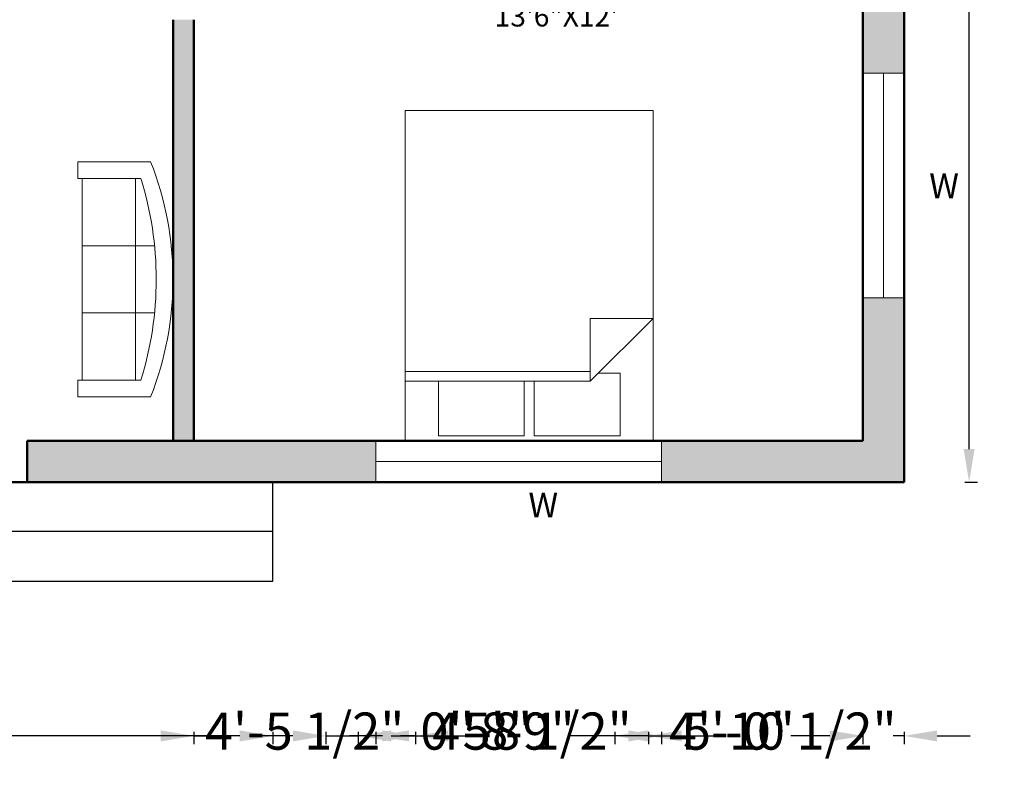
# Model space of a CAD drawing. Units: inches. Extents: x 2568 to 3190, y 746 to 1467.
# Tile 3 of 7: x 2900 to 3139, y 746 to 933. Entities that reach past the tile are written whole.
import ezdxf

# ---------------------------------------------------------------- set-up
doc = ezdxf.new("R2010")
doc.units = ezdxf.units.IN
for name, color, linetype, lineweight in [('A-ANNO-DIMS', 2, 'Continuous', 18), ('A-ANNO-TEXT', 7, 'Continuous', 18), ('A-AREA-IDEN', 7, 'Continuous', 25), ('A-FLOR-STRS', 7, 'Continuous', 25), ('A-FURN', 8, 'Continuous', 18), ('A-GLAZ', 4, 'Continuous', 20), ('A-WALL', 7, 'Continuous', 50), ('A-WALL-PATT', 252, 'Continuous', 13)]:
    doc.layers.add(name, color=color, linetype=linetype, lineweight=lineweight)
doc.styles.get("Standard").update_dxf_attribs({"font": 'arial.ttf'})
doc.dimstyles.new('ISO-25', dxfattribs={"dimtxt": 9, "dimasz": 8, "dimexe": 2, "dimexo": 1, "dimtad": 0, "dimtih": 1, "dimtoh": 1, "dimdec": 1, "dimlunit": 3, "dimtxsty": 'Standard', "dimcen": 2.5, "dimclrd": 1, "dimclre": 3, "dimclrt": 6, "dimadec": 0, "dimazin": 0, "dimtfac": 1, "dimtdec": 1, "dimtmove": 0, "dimatfit": 3, "dimfxl": 1, "dimfxlon": 1, "dimarcsym": 0})

# ---------------------------------------------------------------- blocks, each defined once
blk = doc.blocks.new('Bed - Queen')
for p, q in [((0, -80.00003), (0, 0)), ((0, 0), (59.99999, 0)), ((59.99999, 0), (59.99999, -80.00003)), ((7.99999, -1.2), (28.79998, -1.2)), ((7.99999, -14.4), (7.99999, -1.2)), ((28.79998, -1.2), (28.79998, -14.4)), ((31.19999, -1.2), (51.99999, -1.2)), ((31.19999, -14.4), (31.19999, -1.2)), ((51.99999, -1.2), (51.99999, -16.4)), ((0, -14.4), (44.8, -14.4)), ((59.99999, -29.6), (44.8, -14.4)), ((44.8, -14.4), (44.8, -29.6)), ((51.99999, -16.4), (46.79936, -16.4)), ((44.8, -16.8), (0, -16.8)), ((44.8, -29.6), (59.99999, -29.6)), ((59.99999, -80.00003), (0, -80.00003))]:
    blk.add_line(p, q)
blk = doc.blocks.new('Sofa - Roundback 7 ft.')
for p, q in [((-12.00002, -32.4421), (-12.00003, -6.5971)), ((11.99997, -32.4421), (11.99998, -6.5971)), ((-36.000027, -34), (-36.000027, -11.4696)), ((-35.999844, -13.3819), (35.9998, -13.3819)), ((35.99998, -34), (35.99998, -11.4696)), ((-36.000027, -32.4421), (35.99998, -32.4421))]:
    blk.add_line(p, q)
for points in [[(-36.000027, -34), (-42.000027, -34), (-42.000027, -8)], [(41.99998, -8), (41.99998, -34), (35.99998, -34)]]:
    blk.add_lwpolyline(points)
for centre, radius, start, end in [((0, -114.25), 114.25, 68.43141, 111.5686), ((-0.00001, -127.1968), 121.1968, 72.72033, 107.2797)]:
    blk.add_arc(centre, radius, start, end)
blk = doc.blocks.new('*D14')
at = {"layer": 'A-ANNO-DIMS', "color": 0, "lineweight": -2, "transparency": 16777216}
for p, q in [((3129.28, 1421.35), (3132.28, 1421.35)), ((3130.28, 1413.35), (3130.28, 1126.57)), ((3130.28, 829.35), (3130.28, 1116.13)), ((3129.28, 821.35), (3132.28, 821.35))]:
    blk.add_line(p, q, dxfattribs=at)
at = {"layer": 'A-ANNO-DIMS', "color": 0, "transparency": 16777216}
for points in [[(3128.95, 1413.35), (3131.61, 1413.35), (3130.28, 1421.35)], [(3128.95, 829.35), (3131.61, 829.35), (3130.28, 821.35)]]:
    blk.add_solid(points, dxfattribs=at)
at = {"layer": 'Defpoints', "color": 0, "transparency": 16777216}
for p in [(3114.52, 1421.35), (3114.52, 821.35), (3130.28, 821.35)]:
    blk.add_point(p, dxfattribs=at)
at = {"layer": 'A-ANNO-DIMS', "color": 0, "transparency": 16777216, "insert": (3130.28, 1121.35), "char_height": 9, "attachment_point": 5}
blk.add_mtext("50'", dxfattribs=at)
blk = doc.blocks.new('WIN-BED-LOWER-54.48')
for p, q in [((-5, 54.48), (5, 54.48)), ((0, 0), (0, 54.48)), ((5, 0), (-5, 0))]:
    blk.add_line(p, q)
blk = doc.blocks.new('*D43')
at = {"layer": 'A-ANNO-DIMS', "color": 3, "lineweight": -2, "transparency": 16777216}
for p, q in [((2942.52, 760.85), (2942.52, 757.85)), ((2996.2, 760.85), (2996.2, 757.85))]:
    blk.add_line(p, q, dxfattribs=at)
at = {"layer": 'A-ANNO-DIMS', "color": 1, "lineweight": -2, "transparency": 16777216}
for p, q in [((2934.52, 759.85), (2926.52, 759.85)), ((2942.52, 759.85), (2946.11, 759.85)), ((2996.2, 759.85), (2992.62, 759.85)), ((3004.2, 759.85), (3012.2, 759.85))]:
    blk.add_line(p, q, dxfattribs=at)
at = {"layer": 'A-ANNO-DIMS', "color": 1, "transparency": 16777216}
for points in [[(2934.52, 761.18), (2934.52, 758.51), (2942.52, 759.85)], [(3004.2, 761.18), (3004.2, 758.51), (2996.2, 759.85)]]:
    blk.add_solid(points, dxfattribs=at)
at = {"layer": 'Defpoints', "color": 0, "transparency": 16777216}
for p in [(2942.52, 1411.35), (2996.2, 1411.35), (2996.2, 759.85)]:
    blk.add_point(p, dxfattribs=at)
at = {"layer": 'A-ANNO-DIMS', "color": 6, "transparency": 16777216, "insert": (2969.36, 759.85), "char_height": 9, "attachment_point": 5}
blk.add_mtext('4\'-5 1/2"', dxfattribs=at)
blk = doc.blocks.new('*D44')
at = {"layer": 'A-ANNO-DIMS', "color": 3, "lineweight": -2, "transparency": 16777216}
for p, q in [((2996.2, 760.85), (2996.2, 757.85)), ((3052.64, 760.85), (3052.64, 757.85))]:
    blk.add_line(p, q, dxfattribs=at)
at = {"layer": 'A-ANNO-DIMS', "color": 1, "lineweight": -2, "transparency": 16777216}
for p, q in [((2988.2, 759.85), (2980.2, 759.85)), ((2996.2, 759.85), (3001.17, 759.85)), ((3052.64, 759.85), (3047.67, 759.85)), ((3060.64, 759.85), (3068.64, 759.85))]:
    blk.add_line(p, q, dxfattribs=at)
at = {"layer": 'A-ANNO-DIMS', "color": 1, "transparency": 16777216}
for points in [[(2988.2, 761.18), (2988.2, 758.51), (2996.2, 759.85)], [(3060.64, 761.18), (3060.64, 758.51), (3052.64, 759.85)]]:
    blk.add_solid(points, dxfattribs=at)
at = {"layer": 'Defpoints', "color": 0, "transparency": 16777216}
for p in [(2996.2, 1411.35), (3052.64, 1411.35), (3052.64, 759.85)]:
    blk.add_point(p, dxfattribs=at)
at = {"layer": 'A-ANNO-DIMS', "color": 6, "transparency": 16777216, "insert": (3024.42, 759.85), "char_height": 9, "attachment_point": 5}
blk.add_mtext('4\'-8 1/2"', dxfattribs=at)
blk = doc.blocks.new('*D48')
at = {"layer": 'A-ANNO-DIMS', "color": 3, "lineweight": -2, "transparency": 16777216}
for p, q in [((2986.63, 760.85), (2986.63, 757.85)), ((3055.78, 760.85), (3055.78, 757.85))]:
    blk.add_line(p, q, dxfattribs=at)
at = {"layer": 'A-ANNO-DIMS', "color": 1, "lineweight": -2, "transparency": 16777216}
for p, q in [((2994.63, 759.85), (3008.62, 759.85)), ((3047.78, 759.85), (3033.79, 759.85))]:
    blk.add_line(p, q, dxfattribs=at)
at = {"layer": 'A-ANNO-DIMS', "color": 1, "transparency": 16777216}
for points in [[(2994.63, 761.18), (2994.63, 758.51), (2986.63, 759.85)], [(3047.78, 761.18), (3047.78, 758.51), (3055.78, 759.85)]]:
    blk.add_solid(points, dxfattribs=at)
at = {"layer": 'Defpoints', "color": 0, "transparency": 16777216}
for p in [(2986.63, 821.35), (3055.78, 821.35), (3055.78, 759.85)]:
    blk.add_point(p, dxfattribs=at)
at = {"layer": 'A-ANNO-DIMS', "color": 6, "transparency": 16777216, "insert": (3021.2, 759.85), "char_height": 9, "attachment_point": 5}
blk.add_mtext('5\'-9"', dxfattribs=at)
blk = doc.blocks.new('*D49')
at = {"layer": 'A-ANNO-DIMS', "color": 3, "lineweight": -2, "transparency": 16777216}
for p, q in [((3055.78, 760.85), (3055.78, 757.85)), ((3114.52, 760.85), (3114.52, 757.85))]:
    blk.add_line(p, q, dxfattribs=at)
at = {"layer": 'A-ANNO-DIMS', "color": 1, "lineweight": -2, "transparency": 16777216}
for p, q in [((3047.78, 759.85), (3039.78, 759.85)), ((3055.78, 759.85), (3058.4, 759.85)), ((3114.52, 759.85), (3111.9, 759.85)), ((3122.52, 759.85), (3130.52, 759.85))]:
    blk.add_line(p, q, dxfattribs=at)
at = {"layer": 'A-ANNO-DIMS', "color": 1, "transparency": 16777216}
for points in [[(3047.78, 761.18), (3047.78, 758.51), (3055.78, 759.85)], [(3122.52, 761.18), (3122.52, 758.51), (3114.52, 759.85)]]:
    blk.add_solid(points, dxfattribs=at)
at = {"layer": 'Defpoints', "color": 0, "transparency": 16777216}
for p in [(3055.78, 821.35), (3114.52, 821.35), (3114.52, 759.85)]:
    blk.add_point(p, dxfattribs=at)
at = {"layer": 'A-ANNO-DIMS', "color": 6, "transparency": 16777216, "insert": (3085.15, 759.85), "char_height": 9, "attachment_point": 5}
blk.add_mtext('4\'-10 1/2"', dxfattribs=at)
blk = doc.blocks.new('*D50')
at = {"layer": 'A-ANNO-DIMS', "color": 3, "lineweight": -2, "transparency": 16777216}
for p, q in [((2846.86, 1452.8), (2846.86, 1455.8)), ((2902.21, 1452.8), (2902.21, 1455.8))]:
    blk.add_line(p, q, dxfattribs=at)
at = {"layer": 'A-ANNO-DIMS', "color": 1, "lineweight": -2, "transparency": 16777216}
for p, q in [((2838.86, 1453.8), (2830.86, 1453.8)), ((2846.86, 1453.8), (2851.29, 1453.8)), ((2902.21, 1453.8), (2897.79, 1453.8)), ((2910.21, 1453.8), (2918.21, 1453.8))]:
    blk.add_line(p, q, dxfattribs=at)
at = {"layer": 'A-ANNO-DIMS', "color": 1, "transparency": 16777216}
for points in [[(2838.86, 1455.13), (2838.86, 1452.47), (2846.86, 1453.8)], [(2910.21, 1455.13), (2910.21, 1452.47), (2902.21, 1453.8)]]:
    blk.add_solid(points, dxfattribs=at)
at = {"layer": 'Defpoints', "color": 0, "transparency": 16777216}
for p in [(2902.21, 1453.8), (2846.86, 831.35), (2902.21, 831.35)]:
    blk.add_point(p, dxfattribs=at)
at = {"layer": 'A-ANNO-DIMS', "color": 6, "transparency": 16777216, "insert": (2874.54, 1453.8), "char_height": 9, "attachment_point": 5}
blk.add_mtext('4\'-7 1/2"', dxfattribs=at)
blk = doc.blocks.new('*D51')
at = {"layer": 'A-ANNO-DIMS', "color": 3, "lineweight": -2, "transparency": 16777216}
for p, q in [((2785.87, 760.85), (2785.87, 757.85)), ((2961.66, 760.85), (2961.66, 757.85))]:
    blk.add_line(p, q, dxfattribs=at)
at = {"layer": 'A-ANNO-DIMS', "color": 1, "lineweight": -2, "transparency": 16777216}
for p, q in [((2793.87, 759.85), (2858.1, 759.85)), ((2953.66, 759.85), (2889.42, 759.85))]:
    blk.add_line(p, q, dxfattribs=at)
at = {"layer": 'A-ANNO-DIMS', "color": 1, "transparency": 16777216}
for points in [[(2793.87, 761.18), (2793.87, 758.51), (2785.87, 759.85)], [(2953.66, 761.18), (2953.66, 758.51), (2961.66, 759.85)]]:
    blk.add_solid(points, dxfattribs=at)
at = {"layer": 'Defpoints', "color": 0, "transparency": 16777216}
for p in [(2785.87, 797.35), (2961.66, 797.35), (2961.66, 759.85)]:
    blk.add_point(p, dxfattribs=at)
at = {"layer": 'A-ANNO-DIMS', "color": 6, "transparency": 16777216, "insert": (2873.76, 759.85), "char_height": 9, "attachment_point": 5}
blk.add_mtext('14\'-8"', dxfattribs=at)
blk = doc.blocks.new('*D59')
at = {"layer": 'A-ANNO-DIMS', "color": 3, "lineweight": -2, "transparency": 16777216}
for p, q in [((3044.52, 760.85), (3044.52, 757.85)), ((3104.52, 760.85), (3104.52, 757.85))]:
    blk.add_line(p, q, dxfattribs=at)
at = {"layer": 'A-ANNO-DIMS', "color": 1, "lineweight": -2, "transparency": 16777216}
for p, q in [((3052.52, 759.85), (3061.94, 759.85)), ((3096.52, 759.85), (3087.11, 759.85))]:
    blk.add_line(p, q, dxfattribs=at)
at = {"layer": 'A-ANNO-DIMS', "color": 1, "transparency": 16777216}
for points in [[(3052.52, 761.18), (3052.52, 758.51), (3044.52, 759.85)], [(3096.52, 761.18), (3096.52, 758.51), (3104.52, 759.85)]]:
    blk.add_solid(points, dxfattribs=at)
at = {"layer": 'Defpoints', "color": 0, "transparency": 16777216}
for p in [(3044.52, 1029.35), (3104.52, 1029.35), (3104.52, 759.85)]:
    blk.add_point(p, dxfattribs=at)
at = {"layer": 'A-ANNO-DIMS', "color": 6, "transparency": 16777216, "insert": (3074.52, 759.85), "char_height": 9, "attachment_point": 5}
blk.add_mtext('5\'-0"', dxfattribs=at)
blk = doc.blocks.new('*D60')
at = {"layer": 'A-ANNO-DIMS', "color": 3, "lineweight": -2, "transparency": 16777216}
for p, q in [((2974.52, 760.85), (2974.52, 757.85)), ((2982.36, 760.85), (2982.36, 757.85))]:
    blk.add_line(p, q, dxfattribs=at)
at = {"layer": 'A-ANNO-DIMS', "color": 1, "lineweight": -2, "transparency": 16777216}
for p, q in [((2966.52, 759.85), (2958.52, 759.85)), ((2974.52, 759.85), (2982.36, 759.85)), ((2990.36, 759.85), (2998.36, 759.85))]:
    blk.add_line(p, q, dxfattribs=at)
at = {"layer": 'A-ANNO-DIMS', "color": 1, "transparency": 16777216}
for points in [[(2966.52, 761.18), (2966.52, 758.51), (2974.52, 759.85)], [(2990.36, 761.18), (2990.36, 758.51), (2982.36, 759.85)]]:
    blk.add_solid(points, dxfattribs=at)
at = {"layer": 'Defpoints', "color": 0, "transparency": 16777216}
for p in [(2974.52, 1034.35), (2982.36, 1034.35), (2982.36, 759.85)]:
    blk.add_point(p, dxfattribs=at)
at = {"layer": 'A-ANNO-DIMS', "color": 6, "transparency": 16777216, "insert": (3010.94, 759.85), "char_height": 9, "attachment_point": 5}
blk.add_mtext('0\'-8"', dxfattribs=at)
blk = doc.blocks.new('*D76')
at = {"layer": 'A-ANNO-DIMS', "color": 3, "lineweight": -2, "transparency": 16777216}
for p, q in [((3044.52, 760.85), (3044.52, 757.85)), ((3104.52, 760.85), (3104.52, 757.85))]:
    blk.add_line(p, q, dxfattribs=at)
at = {"layer": 'A-ANNO-DIMS', "color": 1, "lineweight": -2, "transparency": 16777216}
for p, q in [((3052.52, 759.85), (3061.94, 759.85)), ((3096.52, 759.85), (3087.11, 759.85))]:
    blk.add_line(p, q, dxfattribs=at)
at = {"layer": 'A-ANNO-DIMS', "color": 1, "transparency": 16777216}
for points in [[(3052.52, 761.18), (3052.52, 758.51), (3044.52, 759.85)], [(3096.52, 761.18), (3096.52, 758.51), (3104.52, 759.85)]]:
    blk.add_solid(points, dxfattribs=at)
at = {"layer": 'Defpoints', "color": 0, "transparency": 16777216}
for p in [(3044.52, 1202.35), (3104.52, 1202.35), (3104.52, 759.85)]:
    blk.add_point(p, dxfattribs=at)
at = {"layer": 'A-ANNO-DIMS', "color": 6, "transparency": 16777216, "insert": (3074.52, 759.85), "char_height": 9, "attachment_point": 5}
blk.add_mtext('5\'-0"', dxfattribs=at)

msp = doc.modelspace()

# ---------------------------------------------------------------- hatches: boundary and pattern name
at = {"layer": 'A-WALL-PATT'}
h = msp.add_hatch(color=256, dxfattribs=at)
h.dxf.hatch_style = 1
h.paths.add_polyline_path([(2709.74, 1411.35), (2709.74, 1421.35), (2634.52, 1421.35), (2634.52, 1371.08), (2644.52, 1371.08), (2644.52, 1411.35)])
h.paths.add_polyline_path([(2844.66, 1411.35), (2844.66, 1421.35), (2763.78, 1421.35), (2763.78, 1411.35)])
h.paths.add_polyline_path([(2996.2, 1411.35), (2996.2, 1421.35), (2897.43, 1421.35), (2897.43, 1411.35)])
h.paths.add_polyline_path([(3104.52, 1411.35), (3104.52, 1371.08), (3114.52, 1371.08), (3114.52, 1421.35), (3052.64, 1421.35), (3052.64, 1411.35)])
h.paths.add_polyline_path([(3114.52, 1316.62), (3104.52, 1316.62), (3104.52, 1248.37), (3114.52, 1248.37)])
h.paths.add_polyline_path([(3104.52, 1174.04), (3114.52, 1174.04), (3114.52, 1222.08), (3104.52, 1222.08)])
h.paths.add_polyline_path([(3104.52, 1020.11), (3114.52, 1020.11), (3114.52, 1113), (3104.52, 1113)])
h.paths.add_polyline_path([(3104.52, 920.42), (3114.52, 920.42), (3114.52, 992.96), (3104.52, 992.96)])
h.paths.add_polyline_path([(3114.52, 821.35), (3114.52, 865.93), (3104.52, 865.93), (3104.52, 831.35), (3055.78, 831.35), (3055.78, 821.35)])
h.paths.add_polyline_path([(2902.21, 831.35), (2902.21, 821.35), (2986.63, 821.35), (2986.63, 831.35)])
h.paths.add_polyline_path([(2634.52, 821.35), (2676.76, 821.35), (2676.76, 831.35), (2644.52, 831.35), (2644.52, 865.93), (2634.52, 865.93)])
h.paths.add_polyline_path([(2754.37, 821.35), (2846.86, 821.35), (2846.86, 831.35), (2754.37, 831.35)])
h.paths.add_polyline_path([(2644.52, 920.42), (2644.52, 1002.57), (2634.52, 1002.57), (2634.52, 920.42)])
h.paths.add_polyline_path([(2644.52, 1044.16), (2644.52, 1113), (2634.52, 1113), (2634.52, 1044.16)])
h.paths.add_polyline_path([(2644.52, 1248.37), (2644.52, 1316.62), (2634.52, 1316.62), (2634.52, 1248.37)])
h.paths.add_polyline_path([(2634.52, 1222.08), (2634.52, 1174.04), (2644.52, 1174.04), (2644.52, 1222.08)])
h = msp.add_hatch(color=256, dxfattribs=at)
h.dxf.hatch_style = 1
h.paths.add_polyline_path([(2811.52, 1411.35), (2806.52, 1411.35), (2806.52, 1303.35), (2811.52, 1303.35), (2811.52, 1310.35), (2850.52, 1310.35), (2850.52, 1315.35), (2811.52, 1315.35)])
h.paths.add_polyline_path([(2942.52, 1411.35), (2937.52, 1411.35), (2937.52, 1315.35), (2898.52, 1315.35), (2898.52, 1310.35), (2937.52, 1310.35), (2937.52, 1303.35), (2942.52, 1303.35)])
h.paths.add_polyline_path([(2811.52, 1267.35), (2704.52, 1267.35), (2704.52, 1261.35), (2704.52, 1237.35), (2704.52, 1202.35), (2644.52, 1202.35), (2644.52, 1197.35), (2806.52, 1197.35), (2806.52, 1191.38), (2811.52, 1191.38), (2811.52, 1202.35), (2793.52, 1202.35), (2793.52, 1232.35), (2788.52, 1232.35), (2788.52, 1202.35), (2709.52, 1202.35), (2709.52, 1262.35), (2788.52, 1262.35), (2788.52, 1256.35), (2793.52, 1256.35), (2793.52, 1262.35), (2811.52, 1262.35)])
h.paths.add_polyline_path([(2680.52, 1267.35), (2644.52, 1267.35), (2644.52, 1261.35), (2680.52, 1261.35)])
h.paths.add_polyline_path([(3044.52, 1267.35), (2937.52, 1267.35), (2937.52, 1262.35), (2955.52, 1262.35), (2955.52, 1256.35), (2960.52, 1256.35), (2960.52, 1262.35), (3039.52, 1262.35), (3039.52, 1202.35), (2960.52, 1202.35), (2960.52, 1232.35), (2955.52, 1232.35), (2955.52, 1202.35), (2937.52, 1202.35), (2937.52, 1191.38), (2942.52, 1191.38), (2942.52, 1197.35), (3104.52, 1197.35), (3104.52, 1202.35), (3044.52, 1202.35)])
h.paths.add_polyline_path([(3104.52, 1267.35), (3072.52, 1267.35), (3072.52, 1262.35), (3104.52, 1262.35)])
h.paths.add_polyline_path([(2838.1, 1075.35), (2811.52, 1075.35), (2811.52, 1155.35), (2806.52, 1155.35), (2806.52, 1075.35), (2644.52, 1075.35), (2644.52, 1070.35), (2806.52, 1070.35), (2811.52, 1070.35), (2838.1, 1070.35)])
h.paths.add_polyline_path([(3104.52, 1075.35), (2942.52, 1075.35), (2942.52, 1155.38), (2937.52, 1155.38), (2937.52, 1075.35), (2910.92, 1075.35), (2910.92, 1070.35), (2937.52, 1070.35), (3104.52, 1070.35)])
h.paths.add_polyline_path([(2811.52, 1038.35), (2806.52, 1038.35), (2806.52, 980.35), (2644.52, 980.35), (2644.52, 975.35), (2806.52, 975.35), (2806.52, 969.37), (2811.52, 969.37), (2811.52, 975.35)])
h.paths.add_polyline_path([(3104.52, 980.35), (2937.52, 980.35), (2937.52, 969.35), (2942.52, 969.35), (2942.52, 975.35), (3104.52, 975.35)])
h.paths.add_polyline_path([(3104.52, 1034.35), (3039.52, 1034.35), (3039.52, 1004.35), (3044.52, 1004.35), (3044.52, 1029.35), (3104.52, 1029.35)])
h.paths.add_polyline_path([(2942.52, 933.35), (2937.52, 933.35), (2937.52, 831.35), (2942.52, 831.35)])
h.paths.add_polyline_path([(2811.52, 933.37), (2806.52, 933.37), (2806.52, 831.35), (2811.52, 831.35)])

# ---------------------------------------------------------------- linework, layer by layer
at = {"layer": 'A-FLOR-STRS'}
for p, q in [((2961.66, 797.35), (2961.66, 821.35)), ((2961.66, 809.35), (2785.87, 809.35)), ((2785.87, 797.35), (2961.66, 797.35))]:
    msp.add_line(p, q, dxfattribs=at)
at = {"layer": 'A-GLAZ'}
for p, q in [((2986.63, 831.35), (2986.63, 821.35)), ((3055.78, 831.35), (3055.78, 821.35)), ((2986.63, 826.35), (3055.78, 826.35))]:
    msp.add_line(p, q, dxfattribs=at)
at = {"layer": 'A-WALL'}
for p, q in [((3114.52, 821.35), (3114.52, 1421.35)), ((3104.52, 831.35), (3104.52, 1411.35)), ((2937.52, 933.35), (2937.52, 831.35)), ((2942.52, 933.35), (2942.52, 831.35)), ((2902.21, 831.35), (2902.21, 821.35)), ((2902.21, 831.35), (3104.52, 831.35)), ((2634.52, 821.35), (2902.21, 821.35)), ((2902.21, 821.35), (3114.52, 821.35))]:
    msp.add_line(p, q, dxfattribs=at)

# ---------------------------------------------------------------- block references
at = {"layer": 'A-FURN', "xscale": -1, "rotation": 180}
msp.add_blockref('Bed - Queen', (2993.75, 831.35), dxfattribs=at)
at = {"layer": 'A-FURN', "xscale": -0.6782133153273913, "yscale": 0.6782133153273913, "zscale": 0.6782133153273913, "rotation": 270}
msp.add_blockref('Sofa - Roundback 7 ft.', (2937.5, 870.46), dxfattribs=at)
at = {"layer": 'A-GLAZ'}
msp.add_blockref('WIN-BED-LOWER-54.48', (3109.52, 865.93), dxfattribs=at)

# ---------------------------------------------------------------- texts
at = {"layer": 'A-ANNO-TEXT', "char_height": 6, "attachment_point": 1}
for insert in [(3120.62, 896.1), (3023.56, 818.76)]:
    msp.add_mtext_dynamic_manual_height_columns('W', width=7.7602, gutter_width=12.5, heights=[0], dxfattribs=dict(at, insert=insert))
at = {"layer": 'A-AREA-IDEN', "insert": (2995.39, 945.03), "char_height": 5, "attachment_point": 1}
msp.add_mtext_dynamic_manual_height_columns('\\pxqc;BEDROOM\\P13\'6"X12\'', width=69.8646, gutter_width=12.5, heights=[0], dxfattribs=at)

# ---------------------------------------------------------------- dimensions: what is measured, and where the dimension line sits
at = {"layer": 'A-ANNO-DIMS'}
for base, p1, p2, picture, middle in [((2902.2147, 1453.7989), (2846.8636, 831.3489), (2902.2147, 831.3489), '*D50', (2874.5391, 1453.7989)), ((2996.2, 759.85), (2942.52, 1411.35), (2996.2, 1411.35), '*D43', (2969.36, 759.85)), ((3052.64, 759.85), (2996.2, 1411.35), (3052.64, 1411.35), '*D44', (3024.42, 759.85)), ((3104.52, 759.85), (3044.52, 1202.35), (3104.52, 1202.35), '*D76', (3074.52, 759.85)), ((2982.36, 759.85), (2974.52, 1034.35), (2982.36, 1034.35), '*D60', (3010.94, 759.85)), ((3104.52, 759.85), (3044.52, 1029.35), (3104.52, 1029.35), '*D59', (3074.52, 759.85)), ((3055.7816, 759.848), (2986.6252, 821.3489), (3055.7816, 821.3489), '*D48', (3021.2034, 759.848)), ((3114.52, 759.85), (3055.78, 821.35), (3114.52, 821.35), '*D49', (3085.15, 759.85)), ((2961.66, 759.85), (2785.87, 797.35), (2961.66, 797.35), '*D51', (2873.76, 759.85))]:
    dim = msp.add_linear_dim(base=base, p1=p1, p2=p2, dimstyle='ISO-25', override={"dimdec": 1, "dimlfac": 1, "dimrnd": 0, "dimzin": 1, "dimdsep": 46, "dimlunit": 4, "dimfrac": 2}, dxfattribs=at)
    dim.commit()
    dim.dimension.update_dxf_attribs({"geometry": picture, "text_midpoint": middle})
dim = msp.add_linear_dim(base=(3130.28, 821.35), p1=(3114.52, 1421.35), p2=(3114.52, 821.35), angle=90, dimstyle='ISO-25', override={"dimclrd": 0, "dimclre": 0, "dimclrt": 0}, dxfattribs=at)
dim.commit()
dim.dimension.update_dxf_attribs({"geometry": '*D14', "text_midpoint": (3130.28, 1121.35)})

doc.saveas('drawing.dxf')
